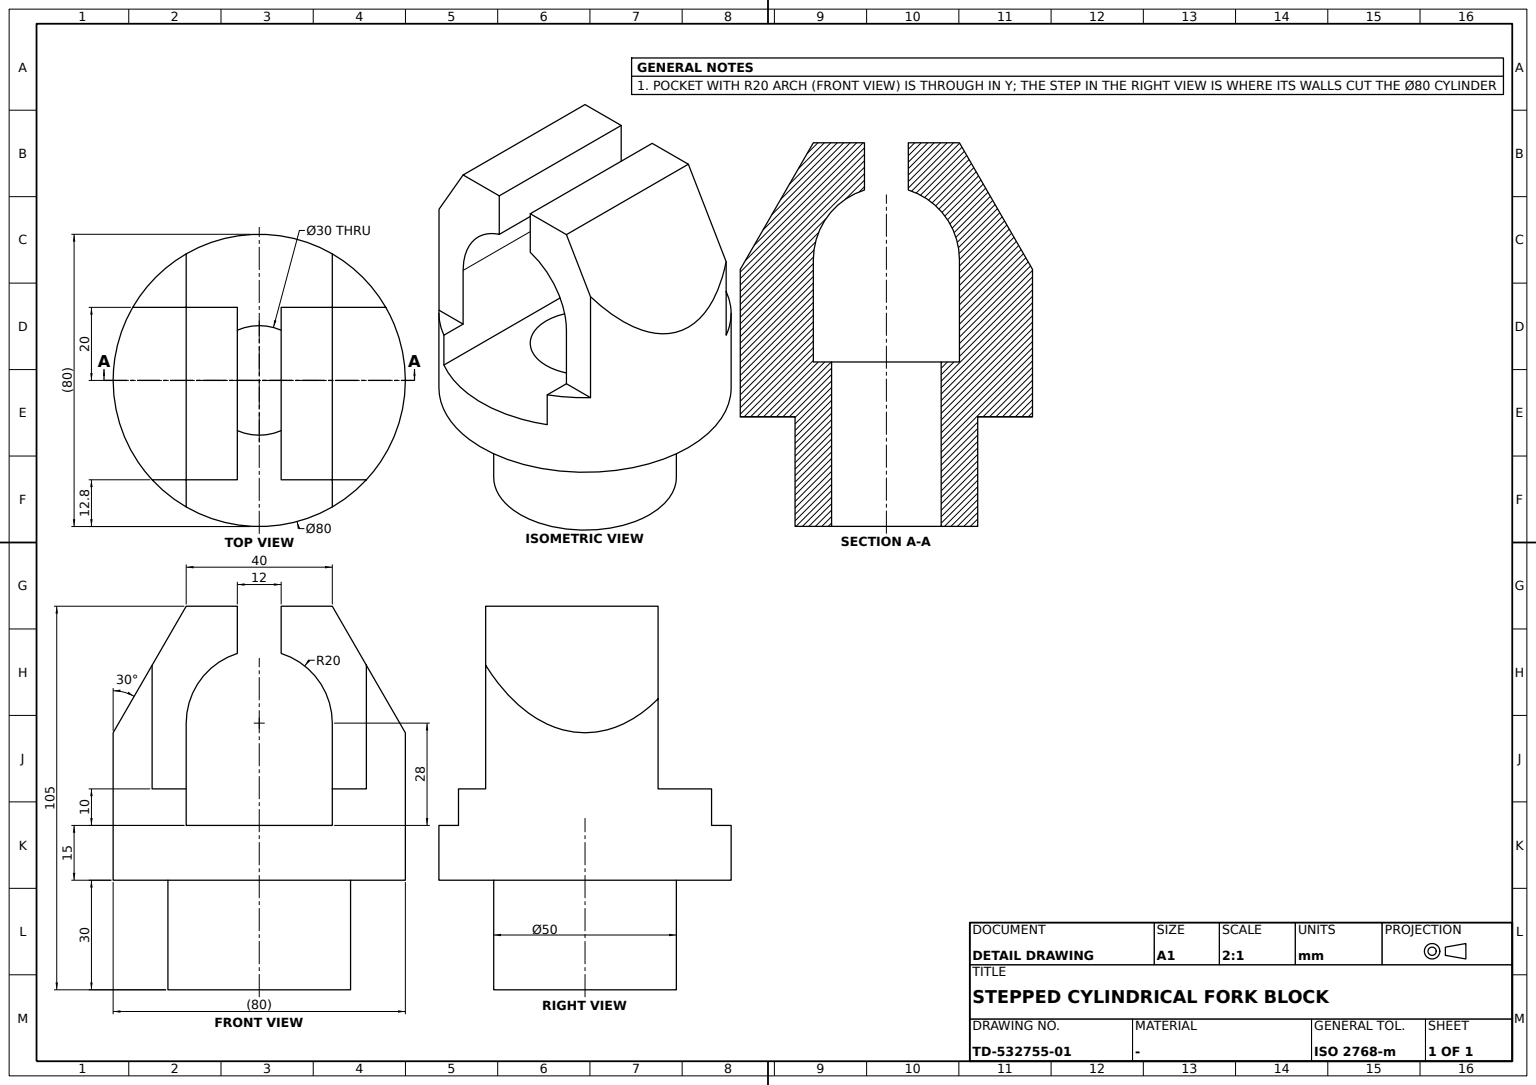
CATIA V5 part; units mm, degrees
sketch "Sketch1" plane through (0, 0, 0) normal (0, 0, 1) x (1, 0, 0)
  circle A0 centre (0, 0) radius 25
  dimension "radius A0" = 25
extrude "Pad1" add sketch "Sketch1" along normal blind 30
sketch "Sketch2" plane through (0, 0, 30) normal (0, 0, 1) x (1, 0, 0)
  circle A0 centre (0, 0) radius 40
  dimension "radius A0" = 40
extrude "Pad2" add sketch "Sketch2" along normal blind 75
sketch "Sketch3" plane through (0, 0, 0) normal (0, 1, 0) x (-1, 0, 0)
  line L0 (-20, 105) -> (-40.2073, 70)
  point P0 (-20, 105)
  point P1 (-40.2073, 70)
  line L1 (-40, 105) -> (40, 105) construction
  line L2 (-40, 30) -> (40, 30) construction
  line L3 (-20, 105) -> (-49.9375, 105)
  line L4 (-49.9375, 105) -> (-49.9375, 53.1468)
  point P2 (-49.9375, 53.1468)
  line L5 (-49.9375, 53.1468) -> (-40.2073, 70)
  dimension "distance P0 y axis" = 20
  dimension "distance P1 L2" = 40
  dimension "D3" = 30
  constraint coincidence P0 L1
  constraint coincidence P2 L0
  constraint horizontal L3 x-axis
  constraint vertical L4 y-axis
  constraint parallelism L5 L0
extrude "Pocket1" cut sketch "Sketch3" along normal mid plane 150
sketch "Sketch4" plane through (0, 0, 0) normal (0, 1, 0) x (-1, 0, 0)
  line L0 (20, 105) -> (63.7934, 29.1476)
  point P0 (20, 105)
  line L1 (-40, 105) -> (40, 105) construction
  line L2 (63.7934, 29.1476) -> (63.7934, 105)
  line L3 (63.7934, 105) -> (20, 105)
  dimension "distance P0 y axis" = 20
  dimension "angle L0 y axis" = 30
  constraint coincidence P0 L1
  constraint vertical L2 y-axis
  constraint horizontal L3 x-axis
extrude "Pocket2" cut sketch "Sketch4" along normal mid plane 150
sketch "Sketch5" plane through (0, 0, 0) normal (1, 0, 0) x (0, 1, 0)
  line L0 (20, 105) -> (20, 55)
  point P0 (20, 105)
  line L1 (-40, 105) -> (40, 105) construction
  line L2 (20, 105) -> (54.2681, 105)
  line L3 (54.2681, 105) -> (54.2681, 55)
  line L4 (54.2681, 55) -> (20, 55)
  dimension "distance L0 y axis" = 20
  dimension "length L0" = 50
  constraint vertical L0 y-axis
  constraint vertical L3 y-axis
  constraint coincidence P0 L1
  constraint horizontal L2 x-axis
  constraint horizontal L4 x-axis
extrude "Pocket3" cut sketch "Sketch5" along normal mid plane 150
sketch "Sketch6" plane through (0, 0, 0) normal (1, 0, 0) x (0, 1, 0)
  line L0 (-27.2017, 105) -> (-27.2017, 55)
  point P0 (-27.2017, 105)
  line L1 (34.641, 105) -> (-34.641, 105) construction
  line L2 (-27.2017, 105) -> (-66.9893, 105)
  line L3 (-66.9893, 105) -> (-66.9893, 55)
  line L4 (-66.9893, 55) -> (-27.2017, 55)
  dimension "length L0" = 50
  constraint vertical L0 y-axis
  constraint vertical L3 y-axis
  constraint coincidence P0 L1
  constraint horizontal L2 x-axis
  constraint horizontal L4 x-axis
extrude "Pocket4" cut sketch "Sketch6" along normal mid plane 150
sketch "Sketch7" plane through (0, 0, 105) normal (0, 0, 1) x (1, 0, 0)
  line L0 (6, 55.0801) -> (6, -55.0801)
  line L1 (6, -55.0801) -> (-6, -55.0801)
  line L2 (-6, -55.0801) -> (-6, 55.0801)
  line L3 (-6, 55.0801) -> (6, 55.0801)
  dimension "length L3" = 12
  constraint vertical L0 y-axis
  constraint vertical L2 y-axis
  constraint horizontal L1 x-axis
  constraint horizontal L3 x-axis
  constraint equidistance L0 L2 origin
  constraint equidistance L1 L3 origin
extrude "Pocket5" cut sketch "Sketch7" against normal blind 40
sketch "Sketch8" plane through (0, 0, 0) normal (0, 1, 0) x (-1, 0, 0)
  line L0 (-20, 73) -> (-20, 45)
  point P0 (-20, 73)
  point P1 (-20, 45)
  line L1 (34.641, 55) -> (-34.641, 55) construction
  line L2 (-20, 105) -> (20, 105) construction
  line L3 (-67.5306, 93) -> (63.2, 93) construction
  arc A0 (20, 73) -> (-20, 73) centre (0, 73) ccw
  point P2 (0, 73)
  point P3 (20, 45)
  point P4 (20, 73)
  line L4 (20, 73) -> (20, 45)
  line L5 (-20, 45) -> (20, 45)
  dimension "distance P1 L1" = 10
  dimension "distance L0 y axis" = 20
  dimension "distance L3 L2" = 12
  constraint vertical L0 y-axis
  constraint horizontal L3 x-axis
  constraint horizontal L5 x-axis
  constraint coincidence P2 y-axis
  constraint tangency A0 L3
  constraint tangency A0 L0
  constraint symmetry P1 P3 y-axis
  constraint symmetry P0 P4 y-axis
  constraint symmetry L0 L4 y-axis
extrude "Pocket6" cut sketch "Sketch8" along normal mid plane 80
sketch "Sketch9" plane through (0, 0, 45) normal (0, 0, 1) x (1, 0, 0)
  circle A0 centre (0, 0) radius 15
  dimension "radius A0" = 15
extrude "Pocket7" cut sketch "Sketch9" against normal through all
